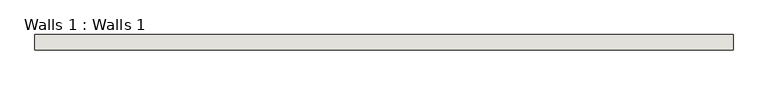
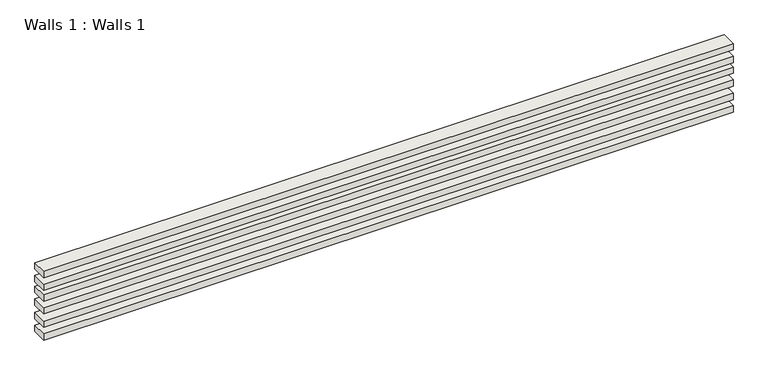
"""IFC4 building model written with IfcOpenShell, lengths in millimetres: wall geometry, Walls 1 : Walls 1."""

from ifc_helpers import new_model, si_unit, frame, origin, place, context, project, spatial, polyline, outline, extrude, source, transform, mapped, element, save


def walls_1_walls_1_ee36d61b(model_context):
    return source(origin(), model_context, "Body", "SweptSolid", [
        extrude(outline(polyline([(3202.9769214, -3274.1217987), (3202.9769214, -3477.3217987), (-5965.6185982, -3477.3217987), (-5965.6185982, -3274.1217987), (3202.9769214, -3274.1217987)])), frame((0.0, 0.0, -57.8232907), z_axis=(0.0, 0.0, 1.0), x_axis=(1.0, 0.0, 0.0)), (0.0, 0.0, 1.0), 88.5693466),
        extrude(outline(polyline([(3202.9769214, -3274.1217987), (3202.9769214, -3477.3217987), (-5965.6185982, -3477.3217987), (-5965.6185982, -3274.1217987), (3202.9769214, -3274.1217987)])), frame((0.0, 0.0, -235.6232907), z_axis=(0.0, 0.0, 1.0), x_axis=(1.0, 0.0, 0.0)), (0.0, 0.0, 1.0), 88.5693466),
        extrude(outline(polyline([(3202.9769214, -3274.1217987), (3202.9769214, -3477.3217987), (-5965.6185982, -3477.3217987), (-5965.6185982, -3274.1217987), (3202.9769214, -3274.1217987)])), frame((0.0, 0.0, -388.0232907), z_axis=(0.0, 0.0, 1.0), x_axis=(1.0, 0.0, 0.0)), (0.0, 0.0, 1.0), 88.5693466),
        extrude(outline(polyline([(3202.9769214, -3274.1217987), (3202.9769214, -3477.3217987), (-5965.6185982, -3477.3217987), (-5965.6185982, -3274.1217987), (3202.9769214, -3274.1217987)])), frame((0.0, 0.0, -565.8232907), z_axis=(0.0, 0.0, 1.0), x_axis=(1.0, 0.0, 0.0)), (0.0, 0.0, 1.0), 88.5693466),
        extrude(outline(polyline([(3202.9769214, -3274.1217987), (3202.9769214, -3477.3217987), (-5965.6185982, -3477.3217987), (-5965.6185982, -3274.1217987), (3202.9769214, -3274.1217987)])), frame((0.0, 0.0, -756.3232907), z_axis=(0.0, 0.0, 1.0), x_axis=(1.0, 0.0, 0.0)), (0.0, 0.0, 1.0), 88.5693466),
        extrude(outline(polyline([(3202.9769214, -3274.1217987), (3202.9769214, -3477.3217987), (-5965.6185982, -3477.3217987), (-5965.6185982, -3274.1217987), (3202.9769214, -3274.1217987)])), frame((0.0, 0.0, -934.1232907), z_axis=(0.0, 0.0, 1.0), x_axis=(1.0, 0.0, 0.0)), (0.0, 0.0, 1.0), 88.5693466),
    ])


if __name__ == "__main__":
    model = new_model("IFC4")
    model_context = context("Model", 3, world=origin())
    ifc_project = project(units=[si_unit("LENGTHUNIT", "METRE", prefix="MILLI")], contexts=[model_context])
    site = spatial("IfcSite", under=ifc_project)
    building = spatial("IfcBuilding", under=site)
    placement = place(None, origin())
    walls_1_walls_1_shape = walls_1_walls_1_ee36d61b(model_context)
    element("IfcWall", 1, ObjectType="Walls 1 : Walls 1", at=placement, inside=building, context=model_context, shape_type="MappedRepresentation", body=[
        mapped(walls_1_walls_1_shape, transform((0.0, 0.0, 0.0), x_axis=(1.0, 0.0, 0.0), y_axis=(0.0, 1.0, 0.0), z_axis=(0.0, 0.0, 1.0))),
    ])
    save(model, "model.ifc")

# Revit data of these elements
# Element 1 (IfcWall, "Walls 1 : Walls 1")
#   Materials on its faces: "Default Wall"
# Materials
#   "Default Wall": colour RGB 128 128 128, transparency 0, Cost = 0
